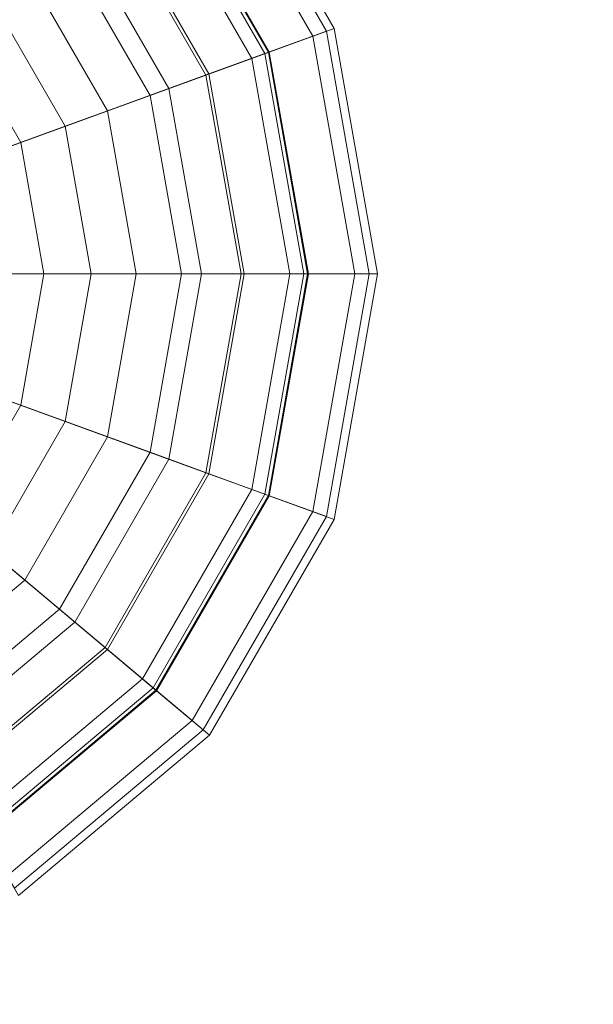
# Model space of a CAD drawing. Units: inches. Extents: x 375 to 1122, y 27 to 1069.
# Tile 59 of 155: x 733.741 to 734.823, y 305.711 to 307.569. Entities that reach past the tile are written whole.
import ezdxf

# ---------------------------------------------------------------- set-up
doc = ezdxf.new("R2010")
doc.units = ezdxf.units.IN
doc.layers.add('A-ANNO-DIMS', color=2, linetype='Continuous', lineweight=18)
doc.layers.add('Furniture', color=30, linetype='Continuous', lineweight=18)
doc.styles.get("Standard").update_dxf_attribs({"font": 'arial.ttf'})
doc.dimstyles.new('ISO-25', dxfattribs={"dimtxt": 12, "dimasz": 2.5, "dimexe": 1.5, "dimexo": 1.5, "dimtad": 1, "dimdec": 1, "dimlunit": 3, "dimtxsty": 'Standard', "dimblk": 'ARCHTICK', "dimcen": 2.5, "dimadec": 0, "dimazin": 0, "dimtfac": 1, "dimtdec": 1, "dimtmove": 0, "dimatfit": 3, "dimfxl": 1.5, "dimfxlon": 1, "dimarcsym": 0})

# ---------------------------------------------------------------- blocks, each defined once
blk = doc.blocks.new('A$C403C54AD')
at = {"linetype": 'ByBlock', "invisible_edges": 5}
for points in [[(1.027872, 1.280047, -0.037345), (1.010941, 1.250721, -0.02811), (1.080205, 1.232162, -0.02811), (1.080205, 1.266024, -0.037345)], [(1.010941, 1.250721, -0.023492), (1.020176, 1.266717, -0.023492), (1.080205, 1.250632, -0.023492), (1.080205, 1.232162, -0.023492)]]:
    blk.add_3dface(points, dxfattribs=at)
at = {"linetype": 'ByBlock'}
blk.add_3dface([(1.010941, 1.250721, -0.02811), (1.010941, 1.250721, -0.023492), (1.080205, 1.232162, -0.023492), (1.080205, 1.232162, -0.02811)], dxfattribs=at)
for points in [[(0.980157, 1.23678, -0.04658), (0.980157, 1.202917, -0.043501), (0.980157, 1.202917, -0.043501), (0.968576, 1.234737, -0.04658)], [(0.980157, 1.233514, -0.043349), (0.980157, 1.23678, -0.04658), (0.968576, 1.234737, -0.04658), (0.969693, 1.231669, -0.043349)], [(0.991739, 1.234737, -0.04658), (0.980157, 1.202917, -0.043501), (0.980157, 1.202917, -0.043501), (0.980157, 1.23678, -0.04658)], [(0.990622, 1.231669, -0.043349), (0.991739, 1.234737, -0.04658), (0.980157, 1.23678, -0.04658), (0.980157, 1.233514, -0.043349)], [(0.980157, 1.233473, 0.116404), (0.980157, 1.236381, 0.10318), (0.968712, 1.234363, 0.10318), (0.969706, 1.231631, 0.116404)], [(0.980157, 1.236381, 0.10318), (0.980157, 1.235706, 0.074938), (0.968943, 1.233728, 0.074938), (0.968712, 1.234363, 0.10318)], [(0.990608, 1.231631, 0.116404), (0.991602, 1.234363, 0.10318), (0.980157, 1.236381, 0.10318), (0.980157, 1.233473, 0.116404)], [(0.991602, 1.234363, 0.10318), (0.991372, 1.233728, 0.074938), (0.980157, 1.235706, 0.074938), (0.980157, 1.236381, 0.10318)], [(0.980157, 1.235706, 0.074938), (0.980157, 1.230341, 0.056929), (0.970778, 1.228687, 0.056929), (0.968943, 1.233728, 0.074938)], [(0.991372, 1.233728, 0.074938), (0.989537, 1.228687, 0.056929), (0.980157, 1.230341, 0.056929), (0.980157, 1.235706, 0.074938)], [(0.968576, 1.234737, -0.04658), (0.980157, 1.202917, -0.043501), (0.980157, 1.202917, -0.043501), (0.958391, 1.228857, -0.04658)], [(0.969693, 1.231669, -0.043349), (0.968576, 1.234737, -0.04658), (0.958391, 1.228857, -0.04658), (0.96049, 1.226356, -0.043349)], [(1.001923, 1.228857, -0.04658), (0.980157, 1.202917, -0.043501), (0.980157, 1.202917, -0.043501), (0.991739, 1.234737, -0.04658)], [(0.999824, 1.226356, -0.043349), (1.001923, 1.228857, -0.04658), (0.991739, 1.234737, -0.04658), (0.990622, 1.231669, -0.043349)], [(0.969706, 1.231631, 0.116404), (0.968712, 1.234363, 0.10318), (0.958647, 1.228552, 0.10318), (0.960516, 1.226325, 0.116404)], [(0.968712, 1.234363, 0.10318), (0.968943, 1.233728, 0.074938), (0.959081, 1.228035, 0.074938), (0.958647, 1.228552, 0.10318)], [(0.999798, 1.226325, 0.116404), (1.001667, 1.228552, 0.10318), (0.991602, 1.234363, 0.10318), (0.990608, 1.231631, 0.116404)], [(1.001667, 1.228552, 0.10318), (1.001233, 1.228035, 0.074938), (0.991372, 1.233728, 0.074938), (0.991602, 1.234363, 0.10318)], [(0.968943, 1.233728, 0.074938), (0.970778, 1.228687, 0.056929), (0.96253, 1.223925, 0.056929), (0.959081, 1.228035, 0.074938)], [(1.001233, 1.228035, 0.074938), (0.997785, 1.223925, 0.056929), (0.989537, 1.228687, 0.056929), (0.991372, 1.233728, 0.074938)], [(0.980157, 1.217132, -0.040074), (0.980157, 1.233514, -0.043349), (0.969693, 1.231669, -0.043349), (0.975296, 1.216274, -0.040074)], [(0.980157, 1.228477, 0.12581), (0.980157, 1.233473, 0.116404), (0.969706, 1.231631, 0.116404), (0.971415, 1.226936, 0.12581)], [(0.980157, 1.233296, 0.102963), (0.980157, 1.230487, 0.115599), (0.970728, 1.228824, 0.115599), (0.969767, 1.231464, 0.102963)], [(0.980157, 1.232638, 0.075423), (0.980157, 1.233296, 0.102963), (0.969767, 1.231464, 0.102963), (0.969992, 1.230846, 0.075423)], [(0.985019, 1.216274, -0.040074), (0.990622, 1.231669, -0.043349), (0.980157, 1.233514, -0.043349), (0.980157, 1.217132, -0.040074)], [(0.988899, 1.226936, 0.12581), (0.990608, 1.231631, 0.116404), (0.980157, 1.233473, 0.116404), (0.980157, 1.228477, 0.12581)], [(0.990547, 1.231464, 0.102963), (0.989586, 1.228824, 0.115599), (0.980157, 1.230487, 0.115599), (0.980157, 1.233296, 0.102963)], [(0.990322, 1.230846, 0.075423), (0.990547, 1.231464, 0.102963), (0.980157, 1.233296, 0.102963), (0.980157, 1.232638, 0.075423)], [(0.980157, 1.227531, 0.058276), (0.980157, 1.232638, 0.075423), (0.969992, 1.230846, 0.075423), (0.971739, 1.226046, 0.058276)], [(0.988575, 1.226046, 0.058276), (0.990322, 1.230846, 0.075423), (0.980157, 1.232638, 0.075423), (0.980157, 1.227531, 0.058276)], [(0.975296, 1.216274, -0.040074), (0.969693, 1.231669, -0.043349), (0.96049, 1.226356, -0.043349), (0.971021, 1.213806, -0.040074)], [(0.971415, 1.226936, 0.12581), (0.969706, 1.231631, 0.116404), (0.960516, 1.226325, 0.116404), (0.963728, 1.222497, 0.12581)], [(0.969767, 1.231464, 0.102963), (0.970728, 1.228824, 0.115599), (0.962436, 1.224037, 0.115599), (0.96063, 1.226189, 0.102963)], [(0.969992, 1.230846, 0.075423), (0.969767, 1.231464, 0.102963), (0.96063, 1.226189, 0.102963), (0.961053, 1.225685, 0.075423)], [(0.989294, 1.213806, -0.040074), (0.999824, 1.226356, -0.043349), (0.990622, 1.231669, -0.043349), (0.985019, 1.216274, -0.040074)], [(0.996587, 1.222497, 0.12581), (0.999798, 1.226325, 0.116404), (0.990608, 1.231631, 0.116404), (0.988899, 1.226936, 0.12581)], [(0.999684, 1.226189, 0.102963), (0.997878, 1.224037, 0.115599), (0.989586, 1.228824, 0.115599), (0.990547, 1.231464, 0.102963)], [(0.999261, 1.225685, 0.075423), (0.999684, 1.226189, 0.102963), (0.990547, 1.231464, 0.102963), (0.990322, 1.230846, 0.075423)], [(0.971739, 1.226046, 0.058276), (0.969992, 1.230846, 0.075423), (0.961053, 1.225685, 0.075423), (0.964336, 1.221772, 0.058276)], [(0.980157, 1.230487, 0.115599), (0.980157, 1.225399, 0.12581), (0.972468, 1.224043, 0.12581), (0.970728, 1.228824, 0.115599)], [(0.989586, 1.228824, 0.115599), (0.987846, 1.224043, 0.12581), (0.980157, 1.225399, 0.12581), (0.980157, 1.230487, 0.115599)], [(0.995978, 1.221772, 0.058276), (0.999261, 1.225685, 0.075423), (0.990322, 1.230846, 0.075423), (0.988575, 1.226046, 0.058276)], [(0.980157, 1.230341, 0.056929), (0.980157, 1.223275, 0.046697), (0.973195, 1.222047, 0.046697), (0.970778, 1.228687, 0.056929)], [(0.989537, 1.228687, 0.056929), (0.98712, 1.222047, 0.046697), (0.980157, 1.223275, 0.046697), (0.980157, 1.230341, 0.056929)], [(0.958391, 1.228857, -0.04658), (0.980157, 1.202917, -0.043501), (0.980157, 1.202917, -0.043501), (0.950832, 1.219849, -0.04658)], [(0.970728, 1.228824, 0.115599), (0.972468, 1.224043, 0.12581), (0.965707, 1.220139, 0.12581), (0.962436, 1.224037, 0.115599)], [(0.970778, 1.228687, 0.056929), (0.973195, 1.222047, 0.046697), (0.967072, 1.218512, 0.046697), (0.96253, 1.223925, 0.056929)], [(1.009483, 1.219849, -0.04658), (0.980157, 1.202917, -0.043501), (0.980157, 1.202917, -0.043501), (1.001923, 1.228857, -0.04658)], [(0.997785, 1.223925, 0.056929), (0.993243, 1.218512, 0.046697), (0.98712, 1.222047, 0.046697), (0.989537, 1.228687, 0.056929)], [(0.997878, 1.224037, 0.115599), (0.994608, 1.220139, 0.12581), (0.987846, 1.224043, 0.12581), (0.989586, 1.228824, 0.115599)], [(1.00662, 1.218195, 0.116404), (1.009137, 1.219649, 0.10318), (1.001667, 1.228552, 0.10318), (0.999798, 1.226325, 0.116404)], [(1.006655, 1.218216, -0.043349), (1.009483, 1.219849, -0.04658), (1.001923, 1.228857, -0.04658), (0.999824, 1.226356, -0.043349)], [(1.009137, 1.219649, 0.10318), (1.008553, 1.219312, 0.074938), (1.001233, 1.228035, 0.074938), (1.001667, 1.228552, 0.10318)], [(0.980157, 1.225399, 0.12581), (0.980157, 1.228477, 0.12581), (0.971415, 1.226936, 0.12581), (0.972468, 1.224043, 0.12581)], [(0.987846, 1.224043, 0.12581), (0.988899, 1.226936, 0.12581), (0.980157, 1.228477, 0.12581), (0.980157, 1.225399, 0.12581)], [(1.008553, 1.219312, 0.074938), (1.003907, 1.216629, 0.056929), (0.997785, 1.223925, 0.056929), (1.001233, 1.228035, 0.074938)], [(0.980157, 1.221045, 0.048884), (0.980157, 1.227531, 0.058276), (0.971739, 1.226046, 0.058276), (0.973957, 1.219951, 0.048884)], [(0.986357, 1.219951, 0.048884), (0.988575, 1.226046, 0.058276), (0.980157, 1.227531, 0.058276), (0.980157, 1.221045, 0.048884)], [(0.972468, 1.224043, 0.12581), (0.971415, 1.226936, 0.12581), (0.963728, 1.222497, 0.12581), (0.965707, 1.220139, 0.12581)], [(0.994608, 1.220139, 0.12581), (0.996587, 1.222497, 0.12581), (0.988899, 1.226936, 0.12581), (0.987846, 1.224043, 0.12581)], [(0.971021, 1.213806, -0.040074), (0.96049, 1.226356, -0.043349), (0.95366, 1.218216, -0.043349), (0.967847, 1.210025, -0.040074)], [(0.992467, 1.210025, -0.040074), (1.006655, 1.218216, -0.043349), (0.999824, 1.226356, -0.043349), (0.989294, 1.213806, -0.040074)], [(1.002293, 1.215697, 0.12581), (1.00662, 1.218195, 0.116404), (0.999798, 1.226325, 0.116404), (0.996587, 1.222497, 0.12581)], [(0.973957, 1.219951, 0.048884), (0.971739, 1.226046, 0.058276), (0.964336, 1.221772, 0.058276), (0.968505, 1.216804, 0.048884)], [(0.991809, 1.216804, 0.048884), (0.995978, 1.221772, 0.058276), (0.988575, 1.226046, 0.058276), (0.986357, 1.219951, 0.048884)], [(1.006466, 1.218107, 0.102963), (1.004033, 1.216702, 0.115599), (0.997878, 1.224037, 0.115599), (0.999684, 1.226189, 0.102963)], [(1.005896, 1.217778, 0.075423), (1.006466, 1.218107, 0.102963), (0.999684, 1.226189, 0.102963), (0.999261, 1.225685, 0.075423)], [(1.001473, 1.215224, 0.058276), (1.005896, 1.217778, 0.075423), (0.999261, 1.225685, 0.075423), (0.995978, 1.221772, 0.058276)], [(1.003907, 1.216629, 0.056929), (0.997787, 1.213096, 0.046697), (0.993243, 1.218512, 0.046697), (0.997785, 1.223925, 0.056929)], [(1.004033, 1.216702, 0.115599), (0.999627, 1.214158, 0.12581), (0.994608, 1.220139, 0.12581), (0.997878, 1.224037, 0.115599)], [(0.980157, 1.223275, 0.046697), (0.980157, 1.213036, 0.03933), (0.976696, 1.212426, 0.03933), (0.973195, 1.222047, 0.046697)], [(0.98712, 1.222047, 0.046697), (0.983618, 1.212426, 0.03933), (0.980157, 1.213036, 0.03933), (0.980157, 1.223275, 0.046697)], [(0.973195, 1.222047, 0.046697), (0.976696, 1.212426, 0.03933), (0.973653, 1.210669, 0.03933), (0.967072, 1.218512, 0.046697)], [(0.993243, 1.218512, 0.046697), (0.986661, 1.210669, 0.03933), (0.983618, 1.212426, 0.03933), (0.98712, 1.222047, 0.046697)], [(0.999627, 1.214158, 0.12581), (1.002293, 1.215697, 0.12581), (0.996587, 1.222497, 0.12581), (0.994608, 1.220139, 0.12581)], [(0.968505, 1.216804, 0.048884), (0.964336, 1.221772, 0.058276), (0.958842, 1.215224, 0.058276), (0.964459, 1.211981, 0.048884)], [(0.995856, 1.211981, 0.048884), (1.001473, 1.215224, 0.058276), (0.995978, 1.221772, 0.058276), (0.991809, 1.216804, 0.048884)], [(0.980157, 1.211822, 0.042248), (0.980157, 1.221045, 0.048884), (0.973957, 1.219951, 0.048884), (0.977112, 1.211285, 0.042248)], [(0.983203, 1.211285, 0.042248), (0.986357, 1.219951, 0.048884), (0.980157, 1.221045, 0.048884), (0.980157, 1.211822, 0.042248)], [(0.977112, 1.211285, 0.042248), (0.973957, 1.219951, 0.048884), (0.968505, 1.216804, 0.048884), (0.974434, 1.209738, 0.042248)], [(0.985881, 1.209738, 0.042248), (0.991809, 1.216804, 0.048884), (0.986357, 1.219951, 0.048884), (0.983203, 1.211285, 0.042248)]]:
    blk.add_3dface(points)
blk = doc.blocks.new('_ArchTick')
at = {"color": 0, "linetype": 'ByBlock', "const_width": 0.15}
blk.add_lwpolyline([(-0.5, -0.5), (0.5, 0.5)], dxfattribs=at)
blk = doc.blocks.new('*D94')
at = {"layer": 'A-ANNO-DIMS', "color": 0, "lineweight": -2, "transparency": 16777216}
for p, q in [((734.0073, 117.5277), (734.0073, 114.5277)), ((773.0073, 117.5277), (773.0073, 114.5277)), ((734.0073, 116.0277), (773.0073, 116.0277))]:
    blk.add_line(p, q, dxfattribs=at)
at = {"layer": 'Defpoints', "color": 0, "transparency": 16777216}
for p in [(734.0073, 667.5277), (773.0073, 667.5277), (773.0073, 116.0277)]:
    blk.add_point(p, dxfattribs=at)
at = {"layer": 'A-ANNO-DIMS', "color": 0, "lineweight": -2, "transparency": 16777216, "xscale": 2.5, "yscale": 2.5, "zscale": 2.5, "rotation": 180}
blk.add_blockref('_ArchTick', (734.0073, 116.0277), dxfattribs=at)
at = {"layer": 'A-ANNO-DIMS', "color": 0, "lineweight": -2, "transparency": 16777216, "xscale": 2.5, "yscale": 2.5, "zscale": 2.5}
blk.add_blockref('_ArchTick', (773.0073, 116.0277), dxfattribs=at)
at = {"layer": 'A-ANNO-DIMS', "color": 0, "transparency": 16777216, "insert": (753.5073, 122.7837), "char_height": 12, "attachment_point": 5}
blk.add_mtext('3\'-3"', dxfattribs=at)

msp = doc.modelspace()

# ---------------------------------------------------------------- block references
at = {"layer": 'Furniture', "xscale": 39.9918517141215, "yscale": 39.9918517141215, "zscale": 39.9918517141215, "rotation": 270}
msp.add_blockref('A$C403C54AD', (684.9549, 346.2875, 0.024), dxfattribs=at)

# ---------------------------------------------------------------- dimensions: what is measured, and where the dimension line sits
at = {"layer": 'A-ANNO-DIMS'}
dim = msp.add_linear_dim(base=(773.0073, 116.0277), p1=(734.0073, 667.5277), p2=(773.0073, 667.5277), dimstyle='ISO-25', override={"dimdec": 1, "dimlfac": 1, "dimrnd": 0, "dimzin": 1, "dimdsep": 46, "dimlunit": 4, "dimfrac": 2}, dxfattribs=at)
dim.commit()
dim.dimension.update_dxf_attribs({"geometry": '*D94', "text_midpoint": (753.5073, 122.7837)})

doc.saveas('drawing.dxf')
